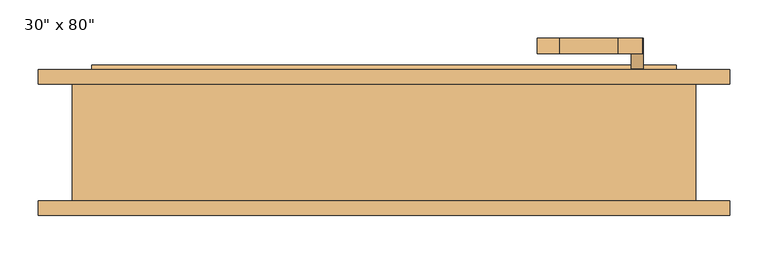
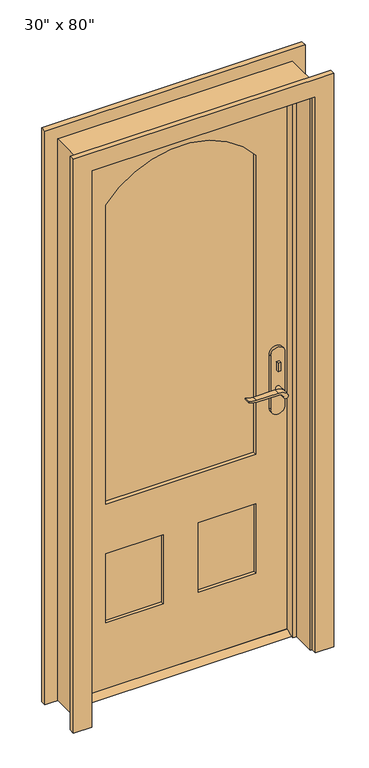
"""IFC4 building model written with IfcOpenShell, lengths in millimetres: door geometry."""

from ifc_helpers import new_model, si_unit, point, frame, frame_2d, origin, place, context, project, spatial, polyline, circle_curve, trimmed, segment, composite_curve, outline, extrude, faceted_brep, source, transform, mapped, element, save


def door_14b9be53(model_context):
    return source(origin(), model_context, "Body", "SolidModel", [
        extrude(outline(polyline([(38.1, 12.7), (73.025, 12.7), (98.425, 0.0), (12.7, 0.0), (38.1, 12.7)])), frame((-381.0, 0.0, 0.0), z_axis=(1.0, 0.0, 0.0), x_axis=(0.0, 1.0, 0.0)), (0.0, 0.0, 1.0), 762.0),
        extrude(outline(polyline([(335.2, 18.1), (325.2, 18.1), (325.2, 28.1), (335.2, 28.1), (335.2, 18.1)])), frame((0.0, 0.0, 981.9), z_axis=(0.0, 0.0, 1.0), x_axis=(1.0, 0.0, 0.0)), (0.0, 0.0, 1.0), 30.0),
        extrude(outline(composite_curve([segment(trimmed(circle_curve(frame_2d((996.9, 330.2)), 8.0), [point((996.9, 322.2))], [point((996.9, 338.2))], False, "CARTESIAN"), True, "CONTINUOUS"), segment(trimmed(circle_curve(frame_2d((996.9, 330.2)), 8.0), [point((996.9, 338.2))], [point((996.9, 322.2))], False, "CARTESIAN"), True, "CONTINUOUS")], self_intersect=False)), frame((0.0, 83.025, 0.0), z_axis=(0.0, 1.0, 0.0), x_axis=(0.0, 0.0, 1.0)), (0.0, 0.0, 1.0), 10.0),
        extrude(outline(composite_curve([segment(trimmed(circle_curve(frame_2d((897.1555521, 306.5324871)), 37.2832219), [point((919.0523287, 336.7081363))], [point((934.4, 304.8325667))], False, "CARTESIAN"), True, "CONTINUOUS"), segment(polyline([(934.4, 304.8325667), (934.4, 228.5564091)]), True, "CONTINUOUS"), segment(trimmed(circle_curve(frame_2d((1017.6850638, 228.6227909)), 83.2850902), [point((934.4, 228.5564091))], [point((939.4, 200.2))], True, "CARTESIAN"), True, "CONTINUOUS"), segment(polyline([(939.4, 200.2), (936.6135558, 200.2)]), True, "CONTINUOUS"), segment(trimmed(circle_curve(frame_2d((986.6709207, 232.1396612)), 59.3791355), [point((936.6135558, 200.2))], [point((927.4, 228.5564091))], False, "CARTESIAN"), True, "CONTINUOUS"), segment(polyline([(927.4, 228.5564091), (927.4, 304.8138099)]), True, "CONTINUOUS"), segment(trimmed(circle_curve(frame_2d((909.2738613, 304.8138099)), 18.1261387), [point((927.4, 304.8138099))], [point((914.4, 322.2))], True, "CARTESIAN"), True, "CONTINUOUS"), segment(trimmed(circle_curve(frame_2d((914.4, 330.2)), 8.0), [point((914.4, 322.2))], [point((919.0523287, 336.7081363))], False, "CARTESIAN"), True, "CONTINUOUS")], self_intersect=False)), frame((0.0, -21.9, 0.0), z_axis=(0.0, 1.0, 0.0), x_axis=(0.0, 0.0, 1.0)), (0.0, 0.0, 1.0), 20.0),
        extrude(outline(composite_curve([segment(trimmed(circle_curve(frame_2d((914.4, 330.2)), 8.0), [point((914.3999903, 322.2))], [point((919.0523287, 336.7081363))], False, "CARTESIAN"), True, "CONTINUOUS"), segment(trimmed(circle_curve(frame_2d((897.1555521, 306.5324871)), 37.2832219), [point((919.0523287, 336.7081363))], [point((934.4, 304.8325667))], False, "CARTESIAN"), True, "CONTINUOUS"), segment(polyline([(934.4, 304.8325667), (934.4, 228.5564091)]), True, "CONTINUOUS"), segment(trimmed(circle_curve(frame_2d((1017.6850638, 228.6227909)), 83.2850902), [point((934.4, 228.5564091))], [point((939.4, 200.2))], True, "CARTESIAN"), True, "CONTINUOUS"), segment(polyline([(939.4, 200.2), (936.6135558, 200.2)]), True, "CONTINUOUS"), segment(trimmed(circle_curve(frame_2d((986.6709207, 232.1396612)), 59.3791355), [point((936.6135558, 200.2))], [point((927.4, 228.5564091))], False, "CARTESIAN"), True, "CONTINUOUS"), segment(polyline([(927.4, 228.5564091), (927.4, 304.8138122)]), True, "CONTINUOUS"), segment(trimmed(circle_curve(frame_2d((909.2738682, 304.8138122)), 18.1261318), [point((927.4, 304.8138122))], [point((914.3999903, 322.2))], True, "CARTESIAN"), True, "CONTINUOUS")], self_intersect=False)), frame((0.0, 113.025, 0.0), z_axis=(0.0, 1.0, 0.0), x_axis=(0.0, 0.0, 1.0)), (0.0, 0.0, 1.0), 20.0),
        extrude(outline(composite_curve([segment(trimmed(circle_curve(frame_2d((914.4, 330.2)), 8.0), [point((914.4, 322.2))], [point((914.4, 338.2))], False, "CARTESIAN"), True, "CONTINUOUS"), segment(trimmed(circle_curve(frame_2d((914.4, 330.2)), 8.0), [point((914.4, 338.2))], [point((914.4, 322.2))], False, "CARTESIAN"), True, "CONTINUOUS")], self_intersect=False)), frame((0.0, -1.9, 0.0), z_axis=(0.0, 1.0, 0.0), x_axis=(0.0, 0.0, 1.0)), (0.0, 0.0, 1.0), 30.0),
        extrude(outline(composite_curve([segment(trimmed(circle_curve(frame_2d((914.4, 330.2)), 8.0), [point((914.4, 322.2))], [point((914.4, 338.2))], False, "CARTESIAN"), True, "CONTINUOUS"), segment(trimmed(circle_curve(frame_2d((914.4, 330.2)), 8.0), [point((914.4, 338.2))], [point((914.4, 322.2))], False, "CARTESIAN"), True, "CONTINUOUS")], self_intersect=False)), frame((0.0, 83.025, 0.0), z_axis=(0.0, 1.0, 0.0), x_axis=(0.0, 0.0, 1.0)), (0.0, 0.0, 1.0), 30.0),
        extrude(outline(composite_curve([segment(polyline([(844.4, 355.2), (1039.4, 355.2)]), True, "CONTINUOUS"), segment(trimmed(circle_curve(frame_2d((1039.4, 330.2)), 25.0), [point((1039.4, 355.2))], [point((1039.4, 305.2))], False, "CARTESIAN"), True, "CONTINUOUS"), segment(polyline([(1039.4, 305.2), (844.4, 305.2)]), True, "CONTINUOUS"), segment(trimmed(circle_curve(frame_2d((844.4, 330.2)), 25.0), [point((844.4, 305.2))], [point((844.4, 355.2))], False, "CARTESIAN"), True, "CONTINUOUS")], self_intersect=False)), frame((0.0, 28.1, 0.0), z_axis=(0.0, 1.0, 0.0), x_axis=(0.0, 0.0, 1.0)), (0.0, 0.0, 1.0), 10.0),
        extrude(outline(composite_curve([segment(polyline([(844.4, 355.2), (1039.4, 355.2)]), True, "CONTINUOUS"), segment(trimmed(circle_curve(frame_2d((1039.4, 330.2)), 25.0), [point((1039.4, 355.2))], [point((1039.4, 305.2))], False, "CARTESIAN"), True, "CONTINUOUS"), segment(polyline([(1039.4, 305.2), (844.4, 305.2)]), True, "CONTINUOUS"), segment(trimmed(circle_curve(frame_2d((844.4, 330.2)), 25.0), [point((844.4, 305.2))], [point((844.4, 355.2))], False, "CARTESIAN"), True, "CONTINUOUS")], self_intersect=False)), frame((0.0, 73.025, 0.0), z_axis=(0.0, 1.0, 0.0), x_axis=(0.0, 0.0, 1.0)), (0.0, 0.0, 1.0), 10.0),
        extrude(outline(polyline([(2032.0, -381.0), (12.7, -381.0), (12.7, 381.0), (2032.0, 381.0), (2032.0, -381.0)]), holes=[composite_curve([segment(polyline([(688.975, -260.35), (1784.35, -260.35)]), True, "CONTINUOUS"), segment(trimmed(circle_curve(frame_2d((1580.99125, 0.0)), 330.35875), [point((1784.35, -260.35))], [point((1784.35, 260.35))], True, "CARTESIAN"), True, "CONTINUOUS"), segment(polyline([(1784.35, 260.35), (688.975, 260.35), (688.975, -260.35)]), True, "CONTINUOUS")], self_intersect=False), polyline([(508.0, -60.325), (254.0, -60.325), (254.0, -260.35), (508.0, -260.35), (508.0, -60.325)]), polyline([(508.0, 260.35), (254.0, 260.35), (254.0, 60.325), (508.0, 60.325), (508.0, 260.35)])]), frame((0.0, 38.1, 0.0), z_axis=(0.0, 1.0, 0.0), x_axis=(0.0, 0.0, 1.0)), (0.0, 0.0, 1.0), 34.925),
        faceted_brep([(406.4, 73.025, 0.0), (406.4, -79.375, 0.0), (381.0, -79.375, 0.0), (381.0, 3.175, 0.0), (368.3, 3.175, 0.0), (368.3, 38.1, 0.0), (381.0, 38.1, 0.0), (381.0, 73.025, 0.0), (406.4, 73.025, 2057.4), (406.4, -79.375, 2057.4), (-406.4, -79.375, 2057.4), (-406.4, -79.375, 0.0), (-381.0, -79.375, 0.0), (-381.0, -79.375, 2032.0), (381.0, -79.375, 2032.0), (381.0, 3.175, 2032.0), (-381.0, 3.175, 2032.0), (-381.0, 3.175, 0.0), (-368.3, 3.175, 0.0), (-368.3, 3.175, 2019.3), (368.3, 3.175, 2019.3), (368.3, 38.1, 2019.3), (-368.3, 38.1, 2019.3), (-368.3, 38.1, 0.0), (-381.0, 38.1, 0.0), (-381.0, 38.1, 2032.0), (381.0, 38.1, 2032.0), (381.0, 73.025, 2032.0), (-381.0, 73.025, 2032.0), (-381.0, 73.025, 0.0), (-406.4, 73.025, 0.0), (-406.4, 73.025, 2057.4)], [[[0, 1, 2, 3, 4, 5, 6, 7]], [[1, 0, 8, 9]], [[2, 1, 9, 10, 11, 12, 13, 14]], [[3, 2, 14, 15]], [[4, 3, 15, 16, 17, 18, 19, 20]], [[5, 4, 20, 21]], [[6, 5, 21, 22, 23, 24, 25, 26]], [[7, 6, 26, 27]], [[0, 7, 27, 28, 29, 30, 31, 8]], [[9, 8, 31, 10]], [[15, 14, 13, 16]], [[21, 20, 19, 22]], [[27, 26, 25, 28]], [[30, 29, 24, 23, 18, 17, 12, 11]], [[10, 31, 30, 11]], [[16, 13, 12, 17]], [[22, 19, 18, 23]], [[28, 25, 24, 29]]]),
        extrude(outline(polyline([(-60.325, 49.7416667), (-260.35, 49.7416667), (-260.35, 61.3833333), (-60.325, 61.3833333), (-60.325, 49.7416667)])), frame((0.0, 0.0, 254.0), z_axis=(0.0, 0.0, 1.0), x_axis=(1.0, 0.0, 0.0)), (0.0, 0.0, 1.0), 254.0),
        extrude(outline(polyline([(260.35, 49.7416667), (60.325, 49.7416667), (60.325, 61.3833333), (260.35, 61.3833333), (260.35, 49.7416667)])), frame((0.0, 0.0, 254.0), z_axis=(0.0, 0.0, 1.0), x_axis=(1.0, 0.0, 0.0)), (0.0, 0.0, 1.0), 254.0),
        extrude(outline(composite_curve([segment(polyline([(688.975, -260.35), (688.975, 260.35), (1784.35, 260.35)]), True, "CONTINUOUS"), segment(trimmed(circle_curve(frame_2d((1580.99125, 0.0)), 330.35875), [point((1784.35, 260.35))], [point((1784.35, -260.35))], False, "CARTESIAN"), True, "CONTINUOUS"), segment(polyline([(1784.35, -260.35), (688.975, -260.35)]), True, "CONTINUOUS")], self_intersect=False)), frame((0.0, 52.07, 0.0), z_axis=(0.0, 1.0, 0.0), x_axis=(0.0, 0.0, 1.0)), (0.0, 0.0, 1.0), 6.985),
        extrude(outline(polyline([(0.0, -450.85), (0.0, -387.35), (2038.35, -387.35), (2038.35, 387.35), (0.0, 387.35), (0.0, 450.85), (2101.85, 450.85), (2101.85, -450.85), (0.0, -450.85)])), frame((0.0, -98.425, 0.0), z_axis=(0.0, 1.0, 0.0), x_axis=(0.0, 0.0, 1.0)), (0.0, 0.0, 1.0), 19.05),
        extrude(outline(polyline([(0.0, -450.85), (0.0, -387.35), (2038.35, -387.35), (2038.35, 387.35), (0.0, 387.35), (0.0, 450.85), (2101.85, 450.85), (2101.85, -450.85), (0.0, -450.85)])), frame((0.0, 73.025, 0.0), z_axis=(0.0, 1.0, 0.0), x_axis=(0.0, 0.0, 1.0)), (0.0, 0.0, 1.0), 19.05),
    ])


if __name__ == "__main__":
    model = new_model("IFC4")
    model_context = context("Model", 3, world=origin())
    ifc_project = project(units=[si_unit("LENGTHUNIT", "METRE", prefix="MILLI")], contexts=[model_context])
    site = spatial("IfcSite", under=ifc_project)
    building = spatial("IfcBuilding", under=site)
    placement = place(None, origin())
    door_shape = door_14b9be53(model_context)
    element("IfcDoor", 1, ObjectType="30\" x 80\"", at=placement, inside=building, context=model_context, shape_type="MappedRepresentation", body=[
        mapped(door_shape, transform((0.0, 0.0, 0.0), x_axis=(1.0, 0.0, 0.0), y_axis=(0.0, 1.0, 0.0), z_axis=(0.0, 0.0, 1.0))),
    ])
    save(model, "model.ifc")

# Revit data of these elements
# Type "30\" x 80\""
#   Type Mark = "10"
#   Assembly Code = "B2030100"
#   Analytic Construction = "French door, wood frame with single glass"
#   Threshold Offset [instance default] = 0' - 0 1/2"
#   Thickness = 0' - 1 3/8"
#   Thermal Resistance (R) = 1.0696 (h·ft²·°F)/BTU
#   Swing Angle [instance default] = 90.00°
#   Stiles = 0' - 4 3/4"
#   Rough Width = 2' - 8"
#   Rough Height = 6' - 9"
#   Radius = 1' - 1.00625"
#   Lock Rail = 0' - 7 1/8"
#   Height = 6' - 8"
#   Width = 2' - 6"
#   Heat Transfer Coefficient (U) = 0.9350 BTU/(h·ft²·°F)
#   Door Offset [instance default] = 0' - 0"
#   Bottom Rail = 0' - 9 1/2"
#   Threshold [instance default] = yes
#   Function = 1
#   Exterior Trim [instance default] = yes
#   Trim Material = Cherry
#   Threshold Material = Cherry
#   Panel Material = Cherry
#   Glazing = Glass
#   Frame Material = Cherry
#   Door Handle Material = Aluminum
#   Visual Light Transmittance = 0
#   Solar Heat Gain Coefficient = 0
#   Wall Closure = (empty or 0)
#   Construction Type = (empty or 0)
# Element 1 (IfcDoor, "30\" x 80\"")
#   Materials on its faces: "Cherry", "Aluminum", "Glass"
# Materials
#   "Cherry": class "Wood", colour RGB 226 177 128, transparency 0, Description = "Prunus Serotina", Cost = 0
#   "Glass": class "Glass", colour RGB 0 128 192, transparency 0.75, Description = "Soda Lime Glass", Cost = 0
#   "Aluminum": class "Metal", colour RGB 247 247 247, transparency 0, Description = "Aluminum 6061", Cost = 0
